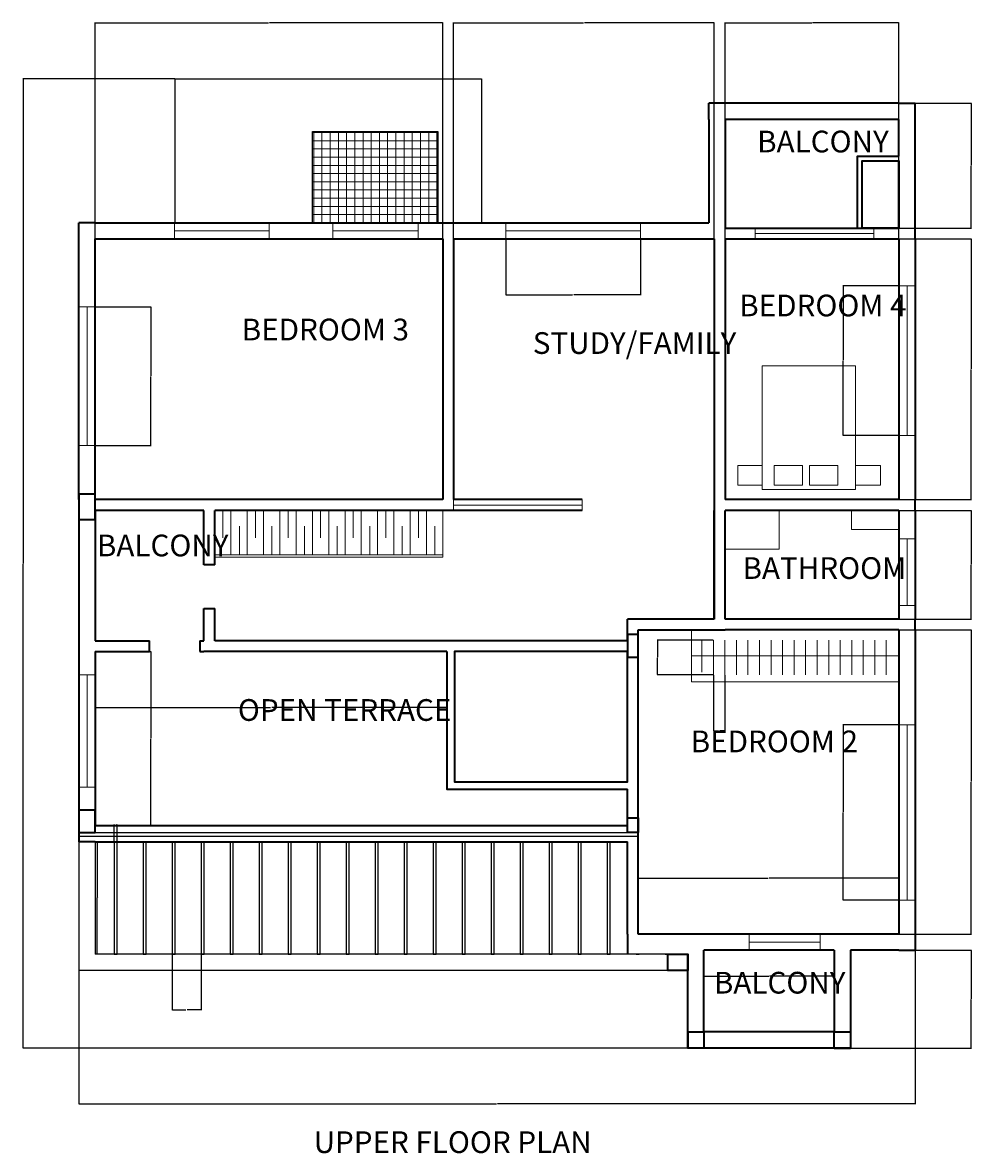
# Model space of a CAD drawing. Units: inches. Extents: x 1741 to 3812, y 9290 to 10023.
# Tile 3 of 5: x 2396 to 2921, y 9307 to 9932. Entities that reach past the tile are written whole.
import ezdxf

# ---------------------------------------------------------------- set-up
doc = ezdxf.new("R2010")
doc.units = ezdxf.units.IN
doc.header["$MEASUREMENT"] = 0
for name, color, linetype, lineweight in [('A-ANNO-DIMS', 2, 'Continuous', 18), ('A-ANNO-TEXT', 7, 'Continuous', 25), ('A-AREA-IDEN', 7, 'Continuous', 18), ('A-COLS', 1, 'Continuous', 35), ('A-FLOR-CASE', 9, 'Continuous', 18), ('A-FLOR-FIXT', 8, 'Continuous', 18), ('A-FLOR-STRS', 3, 'Continuous', 18), ('A-FURN', 9, 'Continuous', 18), ('A-GLAZ', 4, 'Continuous', 18), ('A-ROOF', 7, 'Continuous', 25), ('A-ROOF-PATT', 8, 'Continuous', 13), ('A-WALL', 7, 'Continuous', 35)]:
    doc.layers.add(name, color=color, linetype=linetype, lineweight=lineweight)
doc.styles.get("Standard").update_dxf_attribs({"font": 'arial.ttf'})
doc.dimstyles.get("Standard").update_dxf_attribs({"dimtxt": 0.18, "dimasz": 0.18, "dimexe": 0.18, "dimexo": 0.0625, "dimgap": 0.09, "dimtad": 0, "dimtih": 1, "dimtoh": 1, "dimdec": 4, "dimzin": 0, "dimdsep": 46, "dimtxsty": 'Standard', "dimcen": 0.09, "dimadec": 0, "dimazin": 0, "dimtfac": 1, "dimtdec": 4, "dimtofl": 0, "dimtmove": 0, "dimatfit": 3, "dimfxl": 1, "dimtolj": 1, "dimtzin": 0, "dimarcsym": 0})

# ---------------------------------------------------------------- blocks, each defined once
blk = doc.blocks.new('TERRACE-CANOPY-SLAT')
blk.add_lwpolyline([(0, 0), (1.8, 0), (1.8, 62.15), (0, 62.15)], close=True)
blk = doc.blocks.new('POST-9X9-PLAN')
blk.add_lwpolyline([(9, 0), (0, 0), (0, 9), (9, 9)], close=True)
blk = doc.blocks.new('WARDROBE-HANGER-PLAN')
for q in [(0, 0), (0, 1.59)]:
    blk.add_line((0, 19.29), q)
blk = doc.blocks.new('*D13')
at = {"layer": 'A-ANNO-DIMS', "color": 0, "lineweight": -2, "transparency": 16777216}
for p, q in [((2446.89, 9479.06), (2437.45, 9479.06)), ((2437.63, 9478.88), (2437.63, 9448.17)), ((2437.63, 9417.09), (2437.63, 9447.8)), ((2446.89, 9416.91), (2437.45, 9416.91))]:
    blk.add_line(p, q, dxfattribs=at)
at = {"layer": 'A-ANNO-DIMS', "color": 0, "transparency": 16777216}
for points in [[(2437.6, 9478.88), (2437.66, 9478.88), (2437.63, 9479.06)], [(2437.6, 9417.09), (2437.66, 9417.09), (2437.63, 9416.91)]]:
    blk.add_solid(points, dxfattribs=at)
at = {"layer": 'Defpoints', "color": 0, "transparency": 16777216}
for p in [(2437.63, 9479.06), (2446.95, 9479.06), (2446.95, 9416.91)]:
    blk.add_point(p, dxfattribs=at)
at = {"layer": 'A-ANNO-DIMS', "color": 0, "transparency": 16777216, "insert": (2437.63, 9447.98), "char_height": 0.18, "attachment_point": 5}
blk.add_mtext('\\A1;SLAT 62 TYP.', dxfattribs=at)
blk = doc.blocks.new('*D14')
at = {"layer": 'A-ANNO-DIMS', "color": 0, "lineweight": -2, "transparency": 16777216}
for p, q in [((2446.95, 9479.12), (2446.95, 9488.56)), ((2447.13, 9488.38), (2447.39, 9488.38)), ((2448.56, 9488.38), (2448.31, 9488.38)), ((2448.74, 9479.12), (2448.74, 9488.56))]:
    blk.add_line(p, q, dxfattribs=at)
at = {"layer": 'A-ANNO-DIMS', "color": 0, "transparency": 16777216}
for points in [[(2447.13, 9488.41), (2447.13, 9488.35), (2446.95, 9488.38)], [(2448.56, 9488.41), (2448.56, 9488.35), (2448.74, 9488.38)]]:
    blk.add_solid(points, dxfattribs=at)
at = {"layer": 'Defpoints', "color": 0, "transparency": 16777216}
for p in [(2448.74, 9488.38), (2446.95, 9479.06), (2448.74, 9479.06)]:
    blk.add_point(p, dxfattribs=at)
at = {"layer": 'A-ANNO-DIMS', "color": 0, "transparency": 16777216, "insert": (2447.85, 9488.38), "char_height": 0.18, "attachment_point": 5}
blk.add_mtext('\\A1;2 TYP.', dxfattribs=at)
blk = doc.blocks.new('*D56')
at = {"layer": 'A-ANNO-DIMS', "color": 0, "lineweight": -2, "transparency": 16777216}
for p, q in [((2889.54, 9419), (2889.54, 9334.08)), ((2427.54, 9407.89), (2427.54, 9334.08)), ((2427.72, 9334.26), (2658.25, 9334.26)), ((2889.36, 9334.26), (2658.83, 9334.26))]:
    blk.add_line(p, q, dxfattribs=at)
at = {"layer": 'A-ANNO-DIMS', "color": 0, "transparency": 16777216}
for points in [[(2427.72, 9334.29), (2427.72, 9334.23), (2427.54, 9334.26)], [(2889.36, 9334.29), (2889.36, 9334.23), (2889.54, 9334.26)]]:
    blk.add_solid(points, dxfattribs=at)
at = {"layer": 'Defpoints', "color": 0, "transparency": 16777216}
for p in [(2889.54, 9419.06), (2427.54, 9407.95), (2889.54, 9334.26)]:
    blk.add_point(p, dxfattribs=at)
at = {"layer": 'A-ANNO-DIMS', "color": 0, "transparency": 16777216, "insert": (2658.54, 9334.26), "char_height": 0.18, "attachment_point": 5}
blk.add_mtext('\\A1;462', dxfattribs=at)
blk = doc.blocks.new('*D57')
at = {"layer": 'A-ANNO-DIMS', "color": 0, "lineweight": -2, "transparency": 16777216}
for p, q in [((2480.59, 9900.6), (2396.56, 9900.6)), ((2396.74, 9900.42), (2396.74, 9633.01)), ((2396.74, 9365.24), (2396.74, 9632.65)), ((2763.77, 9365.06), (2396.56, 9365.06))]:
    blk.add_line(p, q, dxfattribs=at)
at = {"layer": 'A-ANNO-DIMS', "color": 0, "transparency": 16777216}
for points in [[(2396.71, 9900.42), (2396.77, 9900.42), (2396.74, 9900.6)], [(2396.71, 9365.24), (2396.77, 9365.24), (2396.74, 9365.06)]]:
    blk.add_solid(points, dxfattribs=at)
at = {"layer": 'Defpoints', "color": 0, "transparency": 16777216}
for p in [(2396.74, 9900.6), (2480.65, 9900.6), (2763.83, 9365.06)]:
    blk.add_point(p, dxfattribs=at)
at = {"layer": 'A-ANNO-DIMS', "color": 0, "transparency": 16777216, "insert": (2396.74, 9632.83), "char_height": 0.18, "attachment_point": 5}
blk.add_mtext('\\A1;535.5', dxfattribs=at)
blk = doc.blocks.new('*D58')
at = {"layer": 'A-ANNO-DIMS', "color": 0, "lineweight": -2, "transparency": 16777216}
for p, q in [((2436.54, 9812.12), (2436.54, 9931.58)), ((2436.72, 9931.4), (2532.26, 9931.4)), ((2628.36, 9931.4), (2532.82, 9931.4)), ((2628.54, 9812.12), (2628.54, 9931.58))]:
    blk.add_line(p, q, dxfattribs=at)
at = {"layer": 'A-ANNO-DIMS', "color": 0, "transparency": 16777216}
for points in [[(2436.72, 9931.43), (2436.72, 9931.37), (2436.54, 9931.4)], [(2628.36, 9931.43), (2628.36, 9931.37), (2628.54, 9931.4)]]:
    blk.add_solid(points, dxfattribs=at)
at = {"layer": 'Defpoints', "color": 0, "transparency": 16777216}
for p in [(2628.54, 9931.4), (2436.54, 9812.06), (2628.54, 9812.06)]:
    blk.add_point(p, dxfattribs=at)
at = {"layer": 'A-ANNO-DIMS', "color": 0, "transparency": 16777216, "insert": (2532.54, 9931.4), "char_height": 0.18, "attachment_point": 5}
blk.add_mtext('\\A1;192', dxfattribs=at)
blk = doc.blocks.new('*D59')
at = {"layer": 'A-ANNO-DIMS', "color": 0, "lineweight": -2, "transparency": 16777216}
for p, q in [((2634.54, 9812.12), (2634.54, 9931.58)), ((2634.72, 9931.4), (2706.26, 9931.4)), ((2778.36, 9931.4), (2706.82, 9931.4)), ((2778.54, 9812.12), (2778.54, 9931.58))]:
    blk.add_line(p, q, dxfattribs=at)
at = {"layer": 'A-ANNO-DIMS', "color": 0, "transparency": 16777216}
for points in [[(2634.72, 9931.43), (2634.72, 9931.37), (2634.54, 9931.4)], [(2778.36, 9931.43), (2778.36, 9931.37), (2778.54, 9931.4)]]:
    blk.add_solid(points, dxfattribs=at)
at = {"layer": 'Defpoints', "color": 0, "transparency": 16777216}
for p in [(2778.54, 9931.4), (2634.54, 9812.06), (2778.54, 9812.06)]:
    blk.add_point(p, dxfattribs=at)
at = {"layer": 'A-ANNO-DIMS', "color": 0, "transparency": 16777216, "insert": (2706.54, 9931.4), "char_height": 0.18, "attachment_point": 5}
blk.add_mtext('\\A1;144', dxfattribs=at)
blk = doc.blocks.new('*D60')
at = {"layer": 'A-ANNO-DIMS', "color": 0, "lineweight": -2, "transparency": 16777216}
for p, q in [((2784.54, 9812.12), (2784.54, 9931.58)), ((2784.72, 9931.4), (2832.32, 9931.4)), ((2880.36, 9931.4), (2832.76, 9931.4)), ((2880.54, 9812.12), (2880.54, 9931.58))]:
    blk.add_line(p, q, dxfattribs=at)
at = {"layer": 'A-ANNO-DIMS', "color": 0, "transparency": 16777216}
for points in [[(2784.72, 9931.43), (2784.72, 9931.37), (2784.54, 9931.4)], [(2880.36, 9931.43), (2880.36, 9931.37), (2880.54, 9931.4)]]:
    blk.add_solid(points, dxfattribs=at)
at = {"layer": 'Defpoints', "color": 0, "transparency": 16777216}
for p in [(2880.54, 9931.4), (2784.54, 9812.06), (2880.54, 9812.06)]:
    blk.add_point(p, dxfattribs=at)
at = {"layer": 'A-ANNO-DIMS', "color": 0, "transparency": 16777216, "insert": (2832.54, 9931.4), "char_height": 0.18, "attachment_point": 5}
blk.add_mtext('\\A1;96', dxfattribs=at)
blk = doc.blocks.new('*D61')
at = {"layer": 'A-ANNO-DIMS', "color": 0, "lineweight": -2, "transparency": 16777216}
for p, q in [((2889.6, 9887.06), (2920.52, 9887.06)), ((2920.34, 9886.88), (2920.34, 9852.74)), ((2920.34, 9818.24), (2920.34, 9852.38)), ((2880.6, 9818.06), (2920.52, 9818.06))]:
    blk.add_line(p, q, dxfattribs=at)
at = {"layer": 'A-ANNO-DIMS', "color": 0, "transparency": 16777216}
for points in [[(2920.31, 9886.88), (2920.37, 9886.88), (2920.34, 9887.06)], [(2920.31, 9818.24), (2920.37, 9818.24), (2920.34, 9818.06)]]:
    blk.add_solid(points, dxfattribs=at)
at = {"layer": 'Defpoints', "color": 0, "transparency": 16777216}
for p in [(2889.54, 9887.06), (2880.54, 9818.06), (2920.34, 9818.06)]:
    blk.add_point(p, dxfattribs=at)
at = {"layer": 'A-ANNO-DIMS', "color": 0, "transparency": 16777216, "insert": (2920.34, 9852.56), "char_height": 0.18, "attachment_point": 5}
blk.add_mtext('\\A1;69', dxfattribs=at)
blk = doc.blocks.new('*D62')
at = {"layer": 'A-ANNO-DIMS', "color": 0, "lineweight": -2, "transparency": 16777216}
for p, q in [((2880.6, 9812.06), (2920.52, 9812.06)), ((2920.34, 9811.88), (2920.34, 9740.24)), ((2920.34, 9668.24), (2920.34, 9739.88)), ((2880.6, 9668.06), (2920.52, 9668.06))]:
    blk.add_line(p, q, dxfattribs=at)
at = {"layer": 'A-ANNO-DIMS', "color": 0, "transparency": 16777216}
for points in [[(2920.31, 9811.88), (2920.37, 9811.88), (2920.34, 9812.06)], [(2920.31, 9668.24), (2920.37, 9668.24), (2920.34, 9668.06)]]:
    blk.add_solid(points, dxfattribs=at)
at = {"layer": 'Defpoints', "color": 0, "transparency": 16777216}
for p in [(2880.54, 9812.06), (2880.54, 9668.06), (2920.34, 9668.06)]:
    blk.add_point(p, dxfattribs=at)
at = {"layer": 'A-ANNO-DIMS', "color": 0, "transparency": 16777216, "insert": (2920.34, 9740.06), "char_height": 0.18, "attachment_point": 5}
blk.add_mtext('\\A1;144', dxfattribs=at)
blk = doc.blocks.new('*D63')
at = {"layer": 'A-ANNO-DIMS', "color": 0, "lineweight": -2, "transparency": 16777216}
for p, q in [((2880.6, 9662.06), (2920.52, 9662.06)), ((2920.34, 9661.88), (2920.34, 9632.24)), ((2920.34, 9602.24), (2920.34, 9631.88)), ((2880.6, 9602.06), (2920.52, 9602.06))]:
    blk.add_line(p, q, dxfattribs=at)
at = {"layer": 'A-ANNO-DIMS', "color": 0, "transparency": 16777216}
for points in [[(2920.31, 9661.88), (2920.37, 9661.88), (2920.34, 9662.06)], [(2920.31, 9602.24), (2920.37, 9602.24), (2920.34, 9602.06)]]:
    blk.add_solid(points, dxfattribs=at)
at = {"layer": 'Defpoints', "color": 0, "transparency": 16777216}
for p in [(2880.54, 9662.06), (2880.54, 9602.06), (2920.34, 9602.06)]:
    blk.add_point(p, dxfattribs=at)
at = {"layer": 'A-ANNO-DIMS', "color": 0, "transparency": 16777216, "insert": (2920.34, 9632.06), "char_height": 0.18, "attachment_point": 5}
blk.add_mtext('\\A1;60', dxfattribs=at)
blk = doc.blocks.new('*D64')
at = {"layer": 'A-ANNO-DIMS', "color": 0, "lineweight": -2, "transparency": 16777216}
for p, q in [((2880.6, 9596.06), (2920.52, 9596.06)), ((2920.34, 9595.88), (2920.34, 9512.24)), ((2920.34, 9428.24), (2920.34, 9511.88)), ((2880.6, 9428.06), (2920.52, 9428.06))]:
    blk.add_line(p, q, dxfattribs=at)
at = {"layer": 'A-ANNO-DIMS', "color": 0, "transparency": 16777216}
for points in [[(2920.31, 9595.88), (2920.37, 9595.88), (2920.34, 9596.06)], [(2920.31, 9428.24), (2920.37, 9428.24), (2920.34, 9428.06)]]:
    blk.add_solid(points, dxfattribs=at)
at = {"layer": 'Defpoints', "color": 0, "transparency": 16777216}
for p in [(2880.54, 9596.06), (2880.54, 9428.06), (2920.34, 9428.06)]:
    blk.add_point(p, dxfattribs=at)
at = {"layer": 'A-ANNO-DIMS', "color": 0, "transparency": 16777216, "insert": (2920.34, 9512.06), "char_height": 0.18, "attachment_point": 5}
blk.add_mtext('\\A1;168', dxfattribs=at)
blk = doc.blocks.new('*D65')
at = {"layer": 'A-ANNO-DIMS', "color": 0, "lineweight": -2, "transparency": 16777216}
for p, q in [((2853.89, 9419.06), (2920.52, 9419.06)), ((2920.34, 9418.88), (2920.34, 9392.24)), ((2920.34, 9365.24), (2920.34, 9391.88)), ((2853.89, 9365.06), (2920.52, 9365.06))]:
    blk.add_line(p, q, dxfattribs=at)
at = {"layer": 'A-ANNO-DIMS', "color": 0, "transparency": 16777216}
for points in [[(2920.31, 9418.88), (2920.37, 9418.88), (2920.34, 9419.06)], [(2920.31, 9365.24), (2920.37, 9365.24), (2920.34, 9365.06)]]:
    blk.add_solid(points, dxfattribs=at)
at = {"layer": 'Defpoints', "color": 0, "transparency": 16777216}
for p in [(2853.83, 9419.06), (2853.83, 9365.06), (2920.34, 9365.06)]:
    blk.add_point(p, dxfattribs=at)
at = {"layer": 'A-ANNO-DIMS', "color": 0, "transparency": 16777216, "insert": (2920.34, 9392.06), "char_height": 0.18, "attachment_point": 5}
blk.add_mtext('\\A1;54', dxfattribs=at)
blk = doc.blocks.new('*D66')
at = {"layer": 'A-ANNO-DIMS', "color": 0, "lineweight": -2, "transparency": 16777216}
for p, q in [((2736.54, 9428.12), (2736.54, 9459.04)), ((2736.72, 9458.86), (2808.26, 9458.86)), ((2880.36, 9458.86), (2808.82, 9458.86)), ((2880.54, 9428.12), (2880.54, 9459.04))]:
    blk.add_line(p, q, dxfattribs=at)
at = {"layer": 'A-ANNO-DIMS', "color": 0, "transparency": 16777216}
for points in [[(2736.72, 9458.89), (2736.72, 9458.83), (2736.54, 9458.86)], [(2880.36, 9458.89), (2880.36, 9458.83), (2880.54, 9458.86)]]:
    blk.add_solid(points, dxfattribs=at)
at = {"layer": 'Defpoints', "color": 0, "transparency": 16777216}
for p in [(2880.54, 9458.86), (2736.54, 9428.06), (2880.54, 9428.06)]:
    blk.add_point(p, dxfattribs=at)
at = {"layer": 'A-ANNO-DIMS', "color": 0, "transparency": 16777216, "insert": (2808.54, 9458.86), "char_height": 0.18, "attachment_point": 5}
blk.add_mtext('\\A1;144', dxfattribs=at)
blk = doc.blocks.new('*D67')
at = {"layer": 'A-ANNO-DIMS', "color": 0, "lineweight": -2, "transparency": 16777216}
for p, q in [((2436.6, 9584.06), (2467.52, 9584.06)), ((2467.34, 9583.88), (2467.34, 9536.24)), ((2467.34, 9488.24), (2467.34, 9535.88)), ((2436.6, 9488.06), (2467.52, 9488.06))]:
    blk.add_line(p, q, dxfattribs=at)
at = {"layer": 'A-ANNO-DIMS', "color": 0, "transparency": 16777216}
for points in [[(2467.31, 9583.88), (2467.37, 9583.88), (2467.34, 9584.06)], [(2467.31, 9488.24), (2467.37, 9488.24), (2467.34, 9488.06)]]:
    blk.add_solid(points, dxfattribs=at)
at = {"layer": 'Defpoints', "color": 0, "transparency": 16777216}
for p in [(2436.54, 9584.06), (2436.54, 9488.06), (2467.34, 9488.06)]:
    blk.add_point(p, dxfattribs=at)
at = {"layer": 'A-ANNO-DIMS', "color": 0, "transparency": 16777216, "insert": (2467.34, 9536.06), "char_height": 0.18, "attachment_point": 5}
blk.add_mtext('\\A1;96', dxfattribs=at)
blk = doc.blocks.new('*D68')
at = {"layer": 'A-ANNO-DIMS', "color": 0, "lineweight": -2, "transparency": 16777216}
for p, q in [((2772.83, 9374.12), (2772.83, 9405.04)), ((2773.01, 9404.86), (2808.61, 9404.86)), ((2844.65, 9404.86), (2809.05, 9404.86)), ((2844.83, 9374.12), (2844.83, 9405.04))]:
    blk.add_line(p, q, dxfattribs=at)
at = {"layer": 'A-ANNO-DIMS', "color": 0, "transparency": 16777216}
for points in [[(2773.01, 9404.89), (2773.01, 9404.83), (2772.83, 9404.86)], [(2844.65, 9404.89), (2844.65, 9404.83), (2844.83, 9404.86)]]:
    blk.add_solid(points, dxfattribs=at)
at = {"layer": 'Defpoints', "color": 0, "transparency": 16777216}
for p in [(2844.83, 9404.86), (2772.83, 9374.06), (2844.83, 9374.06)]:
    blk.add_point(p, dxfattribs=at)
at = {"layer": 'A-ANNO-DIMS', "color": 0, "transparency": 16777216, "insert": (2808.83, 9404.86), "char_height": 0.18, "attachment_point": 5}
blk.add_mtext('\\A1;72', dxfattribs=at)
blk = doc.blocks.new('*D69')
at = {"layer": 'A-ANNO-DIMS', "color": 0, "lineweight": -2, "transparency": 16777216}
for p, q in [((2777.97, 9590.5), (2747.05, 9590.5)), ((2747.23, 9590.32), (2747.23, 9581.03)), ((2747.23, 9571.39), (2747.23, 9580.67)), ((2777.97, 9571.21), (2747.05, 9571.21))]:
    blk.add_line(p, q, dxfattribs=at)
at = {"layer": 'A-ANNO-DIMS', "color": 0, "transparency": 16777216}
for points in [[(2747.2, 9590.32), (2747.26, 9590.32), (2747.23, 9590.5)], [(2747.2, 9571.39), (2747.26, 9571.39), (2747.23, 9571.21)]]:
    blk.add_solid(points, dxfattribs=at)
at = {"layer": 'Defpoints', "color": 0, "transparency": 16777216}
for p in [(2747.23, 9590.5), (2778.03, 9590.5), (2778.03, 9571.21)]:
    blk.add_point(p, dxfattribs=at)
at = {"layer": 'A-ANNO-DIMS', "color": 0, "transparency": 16777216, "insert": (2747.23, 9580.85), "char_height": 0.18, "attachment_point": 5}
blk.add_mtext('\\A1;19.29', dxfattribs=at)
blk = doc.blocks.new('*D70')
at = {"layer": 'A-ANNO-DIMS', "color": 0, "lineweight": -2, "transparency": 16777216}
for p, q in [((2778.03, 9571.15), (2778.03, 9540.23)), ((2784.4, 9571.15), (2784.4, 9540.23)), ((2778.21, 9540.41), (2780.82, 9540.41)), ((2784.22, 9540.41), (2781.61, 9540.41))]:
    blk.add_line(p, q, dxfattribs=at)
at = {"layer": 'A-ANNO-DIMS', "color": 0, "transparency": 16777216}
for points in [[(2778.21, 9540.44), (2778.21, 9540.38), (2778.03, 9540.41)], [(2784.22, 9540.44), (2784.22, 9540.38), (2784.4, 9540.41)]]:
    blk.add_solid(points, dxfattribs=at)
at = {"layer": 'Defpoints', "color": 0, "transparency": 16777216}
for p in [(2778.03, 9571.21), (2784.4, 9571.21), (2778.03, 9540.41)]:
    blk.add_point(p, dxfattribs=at)
at = {"layer": 'A-ANNO-DIMS', "color": 0, "transparency": 16777216, "insert": (2781.21, 9540.41), "char_height": 0.18, "attachment_point": 5}
blk.add_mtext('\\A1;6.369', dxfattribs=at)
blk = doc.blocks.new('*D71')
at = {"layer": 'A-ANNO-DIMS', "color": 0, "lineweight": -2, "transparency": 16777216}
for p, q in [((2478.99, 9416.85), (2478.99, 9385.93)), ((2495.01, 9416.85), (2495.01, 9385.93)), ((2479.17, 9386.11), (2486.61, 9386.11)), ((2494.83, 9386.11), (2487.38, 9386.11))]:
    blk.add_line(p, q, dxfattribs=at)
at = {"layer": 'A-ANNO-DIMS', "color": 0, "transparency": 16777216}
for points in [[(2479.17, 9386.14), (2479.17, 9386.08), (2478.99, 9386.11)], [(2494.83, 9386.14), (2494.83, 9386.08), (2495.01, 9386.11)]]:
    blk.add_solid(points, dxfattribs=at)
at = {"layer": 'Defpoints', "color": 0, "transparency": 16777216}
for p in [(2478.99, 9416.91), (2495.01, 9416.91), (2478.99, 9386.11)]:
    blk.add_point(p, dxfattribs=at)
at = {"layer": 'A-ANNO-DIMS', "color": 0, "transparency": 16777216, "insert": (2487, 9386.11), "char_height": 0.18, "attachment_point": 5}
blk.add_mtext('\\A1;16.02', dxfattribs=at)
blk = doc.blocks.new('*D72')
at = {"layer": 'A-ANNO-DIMS', "color": 0, "lineweight": -2, "transparency": 16777216}
for p, q in [((2436.54, 9584), (2436.54, 9553.08)), ((2630.85, 9584), (2630.85, 9553.08)), ((2436.72, 9553.26), (2533.31, 9553.26)), ((2630.67, 9553.26), (2534.08, 9553.26))]:
    blk.add_line(p, q, dxfattribs=at)
at = {"layer": 'A-ANNO-DIMS', "color": 0, "transparency": 16777216}
for points in [[(2436.72, 9553.29), (2436.72, 9553.23), (2436.54, 9553.26)], [(2630.67, 9553.29), (2630.67, 9553.23), (2630.85, 9553.26)]]:
    blk.add_solid(points, dxfattribs=at)
at = {"layer": 'Defpoints', "color": 0, "transparency": 16777216}
for p in [(2436.54, 9584.06), (2630.85, 9584.06), (2436.54, 9553.26)]:
    blk.add_point(p, dxfattribs=at)
at = {"layer": 'A-ANNO-DIMS', "color": 0, "transparency": 16777216, "insert": (2533.69, 9553.26), "char_height": 0.18, "attachment_point": 5}
blk.add_mtext('\\A1;194.3', dxfattribs=at)
blk = doc.blocks.new('*D73')
at = {"layer": 'A-ANNO-DIMS', "color": 0, "lineweight": -2, "transparency": 16777216}
for p, q in [((2436.6, 9774.48), (2467.52, 9774.48)), ((2467.34, 9774.3), (2467.34, 9736.38)), ((2467.34, 9698.1), (2467.34, 9736.02)), ((2436.6, 9697.92), (2467.52, 9697.92))]:
    blk.add_line(p, q, dxfattribs=at)
at = {"layer": 'A-ANNO-DIMS', "color": 0, "transparency": 16777216}
for points in [[(2467.31, 9774.3), (2467.37, 9774.3), (2467.34, 9774.48)], [(2467.31, 9698.1), (2467.37, 9698.1), (2467.34, 9697.92)]]:
    blk.add_solid(points, dxfattribs=at)
at = {"layer": 'Defpoints', "color": 0, "transparency": 16777216}
for p in [(2436.54, 9774.48), (2436.54, 9697.92), (2467.34, 9697.92)]:
    blk.add_point(p, dxfattribs=at)
at = {"layer": 'A-ANNO-DIMS', "color": 0, "transparency": 16777216, "insert": (2467.34, 9736.2), "char_height": 0.18, "attachment_point": 5}
blk.add_mtext('\\A1;76.57', dxfattribs=at)
blk = doc.blocks.new('*D74')
at = {"layer": 'A-ANNO-DIMS', "color": 0, "lineweight": -2, "transparency": 16777216}
for p, q in [((2663.36, 9812), (2663.36, 9781.08)), ((2737.76, 9812), (2737.76, 9781.08)), ((2663.54, 9781.26), (2700.24, 9781.26)), ((2737.58, 9781.26), (2700.88, 9781.26))]:
    blk.add_line(p, q, dxfattribs=at)
at = {"layer": 'A-ANNO-DIMS', "color": 0, "transparency": 16777216}
for points in [[(2663.54, 9781.29), (2663.54, 9781.23), (2663.36, 9781.26)], [(2737.58, 9781.29), (2737.58, 9781.23), (2737.76, 9781.26)]]:
    blk.add_solid(points, dxfattribs=at)
at = {"layer": 'Defpoints', "color": 0, "transparency": 16777216}
for p in [(2663.36, 9812.06), (2737.76, 9812.06), (2663.36, 9781.26)]:
    blk.add_point(p, dxfattribs=at)
at = {"layer": 'A-ANNO-DIMS', "color": 0, "transparency": 16777216, "insert": (2700.56, 9781.26), "char_height": 0.18, "attachment_point": 5}
blk.add_mtext('\\A1;74.4', dxfattribs=at)
blk = doc.blocks.new('*D75')
at = {"layer": 'A-ANNO-DIMS', "color": 0, "lineweight": -2, "transparency": 16777216}
for p, q in [((2880.48, 9786.2), (2849.56, 9786.2)), ((2849.74, 9786.02), (2849.74, 9745.05)), ((2849.74, 9703.72), (2849.74, 9744.69)), ((2880.48, 9703.54), (2849.56, 9703.54))]:
    blk.add_line(p, q, dxfattribs=at)
at = {"layer": 'A-ANNO-DIMS', "color": 0, "transparency": 16777216}
for points in [[(2849.71, 9786.02), (2849.77, 9786.02), (2849.74, 9786.2)], [(2849.71, 9703.72), (2849.77, 9703.72), (2849.74, 9703.54)]]:
    blk.add_solid(points, dxfattribs=at)
at = {"layer": 'Defpoints', "color": 0, "transparency": 16777216}
for p in [(2849.74, 9786.2), (2880.54, 9786.2), (2880.54, 9703.54)]:
    blk.add_point(p, dxfattribs=at)
at = {"layer": 'A-ANNO-DIMS', "color": 0, "transparency": 16777216, "insert": (2849.74, 9744.87), "char_height": 0.18, "attachment_point": 5}
blk.add_mtext('\\A1;82.66', dxfattribs=at)
blk = doc.blocks.new('*D76')
at = {"layer": 'A-ANNO-DIMS', "color": 0, "lineweight": -2, "transparency": 16777216}
for p, q in [((2880.48, 9543.69), (2849.56, 9543.69)), ((2849.74, 9543.51), (2849.74, 9495.44)), ((2849.74, 9447.01), (2849.74, 9495.08)), ((2880.48, 9446.83), (2849.56, 9446.83))]:
    blk.add_line(p, q, dxfattribs=at)
at = {"layer": 'A-ANNO-DIMS', "color": 0, "transparency": 16777216}
for points in [[(2849.71, 9543.51), (2849.77, 9543.51), (2849.74, 9543.69)], [(2849.71, 9447.01), (2849.77, 9447.01), (2849.74, 9446.83)]]:
    blk.add_solid(points, dxfattribs=at)
at = {"layer": 'Defpoints', "color": 0, "transparency": 16777216}
for p in [(2849.74, 9543.69), (2880.54, 9543.69), (2880.54, 9446.83)]:
    blk.add_point(p, dxfattribs=at)
at = {"layer": 'A-ANNO-DIMS', "color": 0, "transparency": 16777216, "insert": (2849.74, 9495.26), "char_height": 0.18, "attachment_point": 5}
blk.add_mtext('\\A1;96.86', dxfattribs=at)

msp = doc.modelspace()

# ---------------------------------------------------------------- hatches: boundary and pattern name
at = {"layer": 'A-ROOF-PATT'}
h = msp.add_hatch(dxfattribs=at)
h.set_pattern_fill('NET', color=256, scale=36.27322, style=0)
h.paths.add_polyline_path([(2556.6539, 9821.0599), (2625.8165, 9821.0599), (2625.8165, 9871.3807), (2556.6539, 9871.3807)])

# ---------------------------------------------------------------- linework, layer by layer
at = {"layer": 'A-COLS'}
for points in [[(2436.5397, 9671.0807), (2427.5397, 9671.0807), (2427.5397, 9657.1373), (2436.5397, 9657.1373)], [(2736.5397, 9593.6037), (2730.5397, 9593.6037), (2730.5397, 9581.0445), (2736.5397, 9581.0445)], [(2427.5397, 9484.1652), (2436.5397, 9484.1652), (2436.5397, 9496.5144), (2427.5397, 9496.5144)], [(2736.5397, 9484.1652), (2730.5397, 9484.1652), (2730.5397, 9492.1899), (2736.5397, 9492.1899)], [(2752.9474, 9416.9087), (2763.8294, 9416.9087), (2763.8294, 9407.9488), (2752.9474, 9407.9488)]]:
    msp.add_lwpolyline(points, close=True, dxfattribs=at)
at = {"layer": 'A-FLOR-CASE'}
for p, q in [((2771.6603, 9590.4984), (2771.6603, 9572.7985)), ((2873.56, 9590.4984), (2873.56, 9571.2075)), ((2765.8732, 9581.7591), (2880.5397, 9581.7591))]:
    msp.add_line(p, q, dxfattribs=at)
msp.add_lwpolyline([(2880.5397, 9596.0599), (2765.8732, 9596.0599), (2765.8732, 9567.4583), (2880.5397, 9567.4583)], close=True, dxfattribs=at)
at = {"layer": 'A-FLOR-FIXT'}
for points in [[(2784.5397, 9662.0599), (2814.3052, 9662.0599), (2814.3052, 9640.7182), (2784.5397, 9640.7182)], [(2880.5397, 9662.0599), (2854.3687, 9662.0599), (2854.3687, 9651.6074), (2880.5397, 9651.6074)]]:
    msp.add_lwpolyline(points, close=True, dxfattribs=at)
at = {"layer": 'A-FLOR-STRS'}
for p, q in [((2628.5397, 9662.0599), (2502.5397, 9662.0599)), ((2502.5397, 9662.0599), (2502.5397, 9637.5296)), ((2507.0408, 9662.0599), (2507.0408, 9646.8636)), ((2511.5397, 9662.0599), (2511.5397, 9637.5296)), ((2520.5397, 9662.0599), (2520.5397, 9637.5296)), ((2525.0408, 9662.0599), (2525.0408, 9646.8636)), ((2529.5397, 9662.0599), (2529.5397, 9637.5296)), ((2538.5397, 9662.0599), (2538.5397, 9637.5296)), ((2543.0408, 9662.0599), (2543.0408, 9646.8636)), ((2547.5397, 9662.0599), (2547.5397, 9637.5296)), ((2556.5397, 9662.0599), (2556.5397, 9637.5296)), ((2561.0408, 9662.0599), (2561.0408, 9646.8636)), ((2565.5397, 9662.0599), (2565.5397, 9637.5296)), ((2574.5397, 9662.0599), (2574.5397, 9637.5296)), ((2579.0408, 9662.0599), (2579.0408, 9646.8636)), ((2583.5397, 9662.0599), (2583.5397, 9637.5296)), ((2592.5397, 9662.0599), (2592.5397, 9637.5296)), ((2597.0408, 9662.0599), (2597.0408, 9646.8636)), ((2601.5397, 9662.0599), (2601.5397, 9637.5296)), ((2610.5397, 9662.0599), (2610.5397, 9637.5296)), ((2615.0408, 9662.0599), (2615.0408, 9646.8636)), ((2619.5397, 9662.0599), (2619.5397, 9637.5296)), ((2628.5397, 9637.5296), (2628.5397, 9662.0599)), ((2628.5397, 9662.0599), (2628.5397, 9636.2823)), ((2516.1834, 9637.5296), (2516.1834, 9653.3002)), ((2534.1834, 9637.5296), (2534.1834, 9653.3002)), ((2552.1834, 9637.5296), (2552.1834, 9653.3002)), ((2570.1834, 9637.5296), (2570.1834, 9653.3002)), ((2588.1834, 9637.5296), (2588.1834, 9653.3002)), ((2606.1834, 9637.5296), (2606.1834, 9653.3002)), ((2624.1834, 9637.5296), (2624.1834, 9653.3002)), ((2502.5397, 9637.5296), (2628.5397, 9637.5296)), ((2502.5397, 9636.2823), (2628.5397, 9636.2823))]:
    msp.add_line(p, q, dxfattribs=at)
at = {"layer": 'A-FURN'}
for points in [[(2805.0105, 9673.7062), (2856.6166, 9673.7062), (2856.6166, 9741.9619), (2805.0105, 9741.9619)], [(2811.5611, 9676.0539), (2827.3358, 9676.0539), (2827.3358, 9686.9744), (2811.5611, 9686.9744)], [(2831.0387, 9676.0539), (2846.8135, 9676.0539), (2846.8135, 9686.9744), (2831.0387, 9686.9744)]]:
    msp.add_lwpolyline(points, close=True, dxfattribs=at)
for points in [[(2805.0105, 9686.9744), (2791.451, 9686.9744), (2791.451, 9676.0539), (2805.0105, 9676.0539)], [(2856.6166, 9676.0539), (2870.3384, 9676.0539), (2870.3384, 9686.9744), (2856.6166, 9686.9744)]]:
    msp.add_lwpolyline(points, dxfattribs=at)
at = {"layer": 'A-GLAZ'}
for p, q in [((2480.2578, 9816.5599), (2532.5397, 9816.5599)), ((2567.8825, 9816.5599), (2615.0013, 9816.5599)), ((2663.3602, 9816.5599), (2737.7585, 9816.5599)), ((2885.0397, 9703.5403), (2885.0397, 9786.197)), ((2432.0397, 9774.4824), (2432.0397, 9697.9157)), ((2634.5397, 9665.0599), (2705.4442, 9665.0599)), ((2885.0397, 9646.4038), (2885.0397, 9609.5179)), ((2432.0397, 9571.3216), (2432.0397, 9509.1765)), ((2885.0397, 9543.6909), (2885.0397, 9446.8276)), ((2797.7718, 9423.5599), (2836.9401, 9423.5599))]:
    msp.add_line(p, q, dxfattribs=at)
for points in [[(2480.2578, 9821.0599), (2532.5397, 9821.0599), (2532.5397, 9812.0599), (2480.2578, 9812.0599)], [(2615.0013, 9812.0599), (2567.8825, 9812.0599), (2567.8825, 9821.0599), (2615.0013, 9821.0599)], [(2663.3602, 9812.0599), (2737.7585, 9812.0599), (2737.7585, 9821.0599), (2663.3602, 9821.0599)], [(2801.079, 9812.0599), (2866.6472, 9812.0599), (2866.6472, 9818.0599), (2801.079, 9818.0599)], [(2801.079, 9815.0599), (2866.6472, 9815.0599), (2866.6472, 9815.0599), (2801.079, 9815.0599)], [(2889.5397, 9703.5403), (2880.5397, 9703.5403), (2880.5397, 9786.197), (2889.5397, 9786.197)], [(2436.5397, 9697.9157), (2427.5397, 9697.9157), (2427.5397, 9774.4824), (2436.5397, 9774.4824)], [(2634.5397, 9668.0599), (2705.4442, 9668.0599), (2705.4442, 9662.0599), (2634.5397, 9662.0599)], [(2889.5397, 9609.5179), (2880.5397, 9609.5179), (2880.5397, 9646.4038), (2889.5397, 9646.4038)], [(2436.5397, 9509.1765), (2427.5397, 9509.1765), (2427.5397, 9571.3216), (2436.5397, 9571.3216)], [(2889.5397, 9446.8276), (2880.5397, 9446.8276), (2880.5397, 9543.6909), (2889.5397, 9543.6909)], [(2836.9401, 9419.0599), (2797.7718, 9419.0599), (2797.7718, 9428.0599), (2836.9401, 9428.0599)]]:
    msp.add_lwpolyline(points, close=True, dxfattribs=at)
at = {"layer": 'A-ROOF'}
for p, q in [((2556.6539, 9871.3807), (2625.8165, 9871.3807)), ((2556.6539, 9821.0599), (2556.6539, 9871.3807)), ((2625.8165, 9871.3807), (2625.8165, 9821.0599)), ((2625.8165, 9821.0599), (2556.6539, 9821.0599)), ((2427.5397, 9479.0599), (2427.5397, 9407.9488)), ((2436.5397, 9479.0599), (2436.5397, 9416.9087)), ((2763.8294, 9416.9087), (2436.5397, 9416.9087)), ((2763.8294, 9407.9488), (2427.5397, 9407.9488))]:
    msp.add_line(p, q, dxfattribs=at)
for points in [[(2649.888, 9821.0599), (2480.6506, 9821.0599), (2480.6506, 9900.5994), (2649.888, 9900.5994)], [(2427.5397, 9484.1652), (2736.5397, 9484.1652), (2736.5397, 9482.0185), (2427.5397, 9482.0185)]]:
    msp.add_lwpolyline(points, close=True, dxfattribs=at)
for points in [[(2735.2955, 9416.9087), (2735.2955, 9416.9087), (2737.0921, 9416.9087)], [(2751.3147, 9416.9087), (2751.3147, 9416.9087), (2753.1114, 9416.9087)]]:
    msp.add_lwpolyline(points, dxfattribs=at)
at = {"layer": 'A-WALL'}
for p, q in [((2775.5397, 9878.0599), (2775.5397, 9887.0599)), ((2784.5397, 9887.0599), (2775.5397, 9887.0599)), ((2880.5397, 9887.0599), (2784.5397, 9887.0599)), ((2880.5397, 9887.0599), (2889.5397, 9887.0599)), ((2889.5397, 9878.0599), (2889.5397, 9887.0599)), ((2775.5397, 9878.0599), (2775.5397, 9821.0599)), ((2880.5397, 9878.0599), (2784.5397, 9878.0599)), ((2784.5397, 9878.0599), (2784.5397, 9818.0599)), ((2880.5397, 9857.8827), (2880.5397, 9878.0599)), ((2889.5397, 9818.0599), (2889.5397, 9878.0599)), ((2880.5397, 9818.0599), (2880.5397, 9855.273)), ((2436.5397, 9821.0599), (2427.5397, 9821.0599)), ((2427.5397, 9812.0599), (2427.5397, 9821.0599)), ((2436.5397, 9821.0599), (2775.5397, 9821.0599)), ((2634.5397, 9821.0599), (2775.5397, 9821.0599)), ((2784.5397, 9818.0599), (2880.5397, 9818.0599)), ((2889.5397, 9812.0599), (2889.5397, 9818.0599)), ((2427.5397, 9668.0599), (2427.5397, 9812.0599)), ((2436.5397, 9812.0599), (2628.5397, 9812.0599)), ((2436.5397, 9668.0599), (2436.5397, 9812.0599)), ((2628.5397, 9812.0599), (2628.5397, 9668.0599)), ((2634.5397, 9812.0599), (2634.5397, 9668.0599)), ((2634.5397, 9812.0599), (2778.5397, 9812.0599)), ((2778.5397, 9812.0599), (2778.5397, 9602.0599)), ((2784.5397, 9812.0599), (2784.5397, 9668.0599)), ((2784.5397, 9812.0599), (2880.5397, 9812.0599)), ((2880.5397, 9812.0599), (2880.5397, 9668.0599)), ((2889.5397, 9812.0599), (2889.5397, 9668.0599)), ((2427.5397, 9668.0599), (2427.5397, 9662.0599)), ((2628.5397, 9668.0599), (2436.5397, 9668.0599)), ((2705.4442, 9668.0599), (2634.5397, 9668.0599)), ((2880.5397, 9668.0599), (2784.5397, 9668.0599)), ((2889.5397, 9662.0599), (2889.5397, 9668.0599)), ((2427.5397, 9662.0599), (2427.5397, 9590.0599)), ((2436.5397, 9662.0599), (2436.5397, 9590.0599)), ((2496.5397, 9662.0599), (2436.5397, 9662.0599)), ((2496.5397, 9631.9948), (2496.5397, 9662.0599)), ((2628.5397, 9662.0599), (2502.5397, 9662.0599)), ((2705.4442, 9662.0599), (2502.5397, 9662.0599)), ((2502.5397, 9631.9948), (2502.5397, 9662.0599)), ((2778.5397, 9602.0599), (2778.5397, 9662.0599)), ((2880.5397, 9662.0599), (2784.5397, 9662.0599)), ((2784.5397, 9602.0599), (2784.5397, 9662.0599)), ((2880.5397, 9662.0599), (2880.5397, 9602.0599)), ((2889.5397, 9662.0599), (2889.5397, 9602.0599)), ((2496.5397, 9590.0599), (2496.5397, 9607.9205)), ((2502.5397, 9590.0599), (2502.5397, 9607.9205)), ((2730.5397, 9590.0599), (2730.5397, 9602.0599)), ((2778.5397, 9602.0599), (2730.5397, 9602.0599)), ((2880.5397, 9602.0599), (2784.5397, 9602.0599)), ((2889.5397, 9596.0599), (2889.5397, 9602.0599)), ((2736.5397, 9428.0599), (2736.5397, 9596.0599)), ((2736.5397, 9596.0599), (2784.5397, 9596.0599)), ((2880.5397, 9596.0599), (2784.5397, 9596.0599)), ((2880.5397, 9596.0599), (2880.5397, 9428.0599)), ((2889.5397, 9596.0599), (2889.5397, 9428.0599)), ((2427.5397, 9590.0599), (2427.5397, 9584.0599)), ((2436.5397, 9590.0599), (2466.5397, 9590.0599)), ((2494.3167, 9590.0599), (2496.5397, 9590.0599)), ((2730.5397, 9590.0599), (2502.5397, 9590.0599)), ((2427.5397, 9584.0599), (2427.5397, 9488.0599)), ((2436.5397, 9584.0599), (2466.5397, 9584.0599)), ((2436.5397, 9584.0599), (2436.5397, 9488.0599)), ((2494.3167, 9584.0599), (2496.5397, 9584.0599)), ((2630.8472, 9584.0599), (2496.5397, 9584.0599)), ((2730.5397, 9584.0599), (2635.0071, 9584.0599)), ((2730.5397, 9512.1654), (2730.5397, 9584.0599)), ((2730.5397, 9488.0599), (2730.5397, 9508.0055)), ((2427.5397, 9488.0599), (2427.5397, 9479.0599)), ((2436.5397, 9488.0599), (2730.5397, 9488.0599)), ((2436.5397, 9479.0599), (2427.5397, 9479.0599)), ((2436.5397, 9479.0599), (2730.5397, 9479.0599)), ((2730.5397, 9428.0599), (2730.5397, 9479.0599)), ((2730.5397, 9428.0599), (2730.5397, 9416.9087)), ((2880.5397, 9428.0599), (2736.5397, 9428.0599)), ((2889.5397, 9428.0599), (2889.5397, 9419.0599)), ((2763.8294, 9374.0599), (2763.8294, 9416.9087)), ((2772.8294, 9374.0599), (2772.8294, 9419.0599)), ((2844.8294, 9419.0599), (2772.8294, 9419.0599)), ((2844.8294, 9419.0599), (2844.8294, 9374.0599)), ((2853.8294, 9419.0599), (2853.8294, 9374.0599)), ((2880.5397, 9419.0599), (2853.8294, 9419.0599)), ((2880.5397, 9419.0599), (2889.5397, 9419.0599)), ((2763.8294, 9374.0599), (2763.8294, 9365.0599)), ((2844.8294, 9374.0599), (2772.8294, 9374.0599)), ((2853.8294, 9374.0599), (2853.8294, 9365.0599)), ((2772.8294, 9365.0599), (2763.8294, 9365.0599)), ((2844.8294, 9365.0599), (2772.8294, 9365.0599)), ((2844.8294, 9365.0599), (2853.8294, 9365.0599))]:
    msp.add_line(p, q, dxfattribs=at)
for points in [[(2857.6888, 9818.0599), (2857.6888, 9857.8827), (2880.5397, 9857.8827)], [(2502.5397, 9631.9948), (2496.5397, 9631.9948)], [(2496.5397, 9607.9205), (2502.5397, 9607.9205)], [(2466.5397, 9584.0599), (2466.5397, 9590.0599)], [(2494.3167, 9590.0599), (2494.3167, 9584.0599)], [(2630.8472, 9584.0599), (2630.8472, 9508.0055), (2730.5397, 9508.0055)]]:
    msp.add_lwpolyline(points, dxfattribs=at)
for points in [[(2880.5397, 9818.0599), (2860.2985, 9818.0599), (2860.2985, 9855.273), (2880.5397, 9855.273)], [(2730.5397, 9584.0599), (2635.0071, 9584.0599), (2635.0071, 9512.1654), (2730.5397, 9512.1654)]]:
    msp.add_lwpolyline(points, close=True, dxfattribs=at)

# ---------------------------------------------------------------- block references
at = {"layer": 'A-COLS'}
for p, rotation in [((2772.8291, 9365.0597), 90.00000000000479), ((2853.8295, 9374.0596), 180)]:
    msp.add_blockref('POST-9X9-PLAN', p, dxfattribs=dict(at, rotation=rotation))
at = {"layer": 'A-FLOR-CASE'}
for p in [(2778.029, 9571.208), (2784.3977, 9571.208), (2790.7665, 9571.208), (2797.1352, 9571.208), (2803.5039, 9571.208), (2809.8727, 9571.208), (2816.2414, 9571.208), (2822.6101, 9571.208), (2828.9789, 9571.208), (2835.3476, 9571.208), (2841.7163, 9571.208), (2848.0851, 9571.208), (2854.4538, 9571.208), (2860.8226, 9571.208), (2867.1913, 9571.208)]:
    msp.add_blockref('WARDROBE-HANGER-PLAN', p, dxfattribs=at)
at = {"layer": 'A-ROOF'}
for p in [(2446.948, 9416.909), (2462.9673, 9416.909), (2478.9866, 9416.909), (2495.0059, 9416.909), (2511.0251, 9416.909), (2527.0444, 9416.909), (2543.0637, 9416.909), (2559.083, 9416.909), (2575.1023, 9416.909), (2591.1216, 9416.909), (2607.1409, 9416.909), (2623.1602, 9416.909), (2639.1794, 9416.909), (2655.1987, 9416.909), (2671.218, 9416.909), (2687.2373, 9416.909), (2703.2566, 9416.909), (2719.2759, 9416.909)]:
    msp.add_blockref('TERRACE-CANOPY-SLAT', p, dxfattribs=at)

# ---------------------------------------------------------------- texts
at = {"layer": 'A-ANNO-TEXT'}
msp.add_text('UPPER FLOOR PLAN', height=12, dxfattribs=at).set_placement((2557.2179, 9307.093))
at = {"layer": 'A-AREA-IDEN'}
for s, p in [('BALCONY', (2802.1816, 9859.8778)), ('BEDROOM 4', (2792.3074, 9769.2958)), ('BEDROOM 3 ', (2517.4793, 9756.0136)), ('STUDY/FAMILY', (2678.2744, 9748.5536)), ('BALCONY ', (2437.4666, 9636.7207)), ('BATHROOM', (2794.1109, 9624.2277)), ('OPEN TERRACE', (2515.3432, 9545.8302)), ('BEDROOM 2', (2765.5039, 9528.4666)), ('BALCONY', (2778.2937, 9395.1731))]:
    msp.add_text(s, height=12, dxfattribs=at).set_placement(p)

# ---------------------------------------------------------------- dimensions: what is measured, and where the dimension line sits
at = {"layer": 'A-ANNO-DIMS'}
for base, p1, p2, picture, middle in [((2628.5397, 9931.3994), (2436.5397, 9812.0599), (2628.5397, 9812.0599), '*D58', (2532.5397, 9931.3994)), ((2778.5397, 9931.3994), (2634.5397, 9812.0599), (2778.5397, 9812.0599), '*D59', (2706.5397, 9931.3994)), ((2880.5397, 9931.3994), (2784.5397, 9812.0599), (2880.5397, 9812.0599), '*D60', (2832.5397, 9931.3994)), ((2880.5397, 9458.8599), (2736.5397, 9428.0599), (2880.5397, 9428.0599), '*D66', (2808.5397, 9458.8599)), ((2889.5397, 9334.2599), (2427.5397, 9407.9488), (2889.5397, 9419.0599), '*D56', (2658.5397, 9334.2599)), ((2844.8294, 9404.8599), (2772.8294, 9374.0599), (2844.8294, 9374.0599), '*D68', (2808.8294, 9404.8599))]:
    dim = msp.add_linear_dim(base=base, p1=p1, p2=p2, dimstyle='Standard', override={"dimdec": 0, "dimlfac": 1, "dimrnd": 0, "dimzin": 0, "dimdsep": 46, "dimlunit": 2}, dxfattribs=at)
    dim.commit()
    dim.dimension.update_dxf_attribs({"geometry": picture, "text_midpoint": middle})
for base, p1, p2, angle, override, picture, middle in [((2396.7397, 9900.5994), (2763.8294, 9365.0599), (2480.6506, 9900.5994), 90, {"dimdec": 1, "dimlfac": 1, "dimrnd": 0, "dimzin": 0, "dimdsep": 46, "dimlunit": 2}, '*D57', (2396.7397, 9632.8297)), ((2920.3397, 9818.0599), (2889.5397, 9887.0599), (2880.5397, 9818.0599), 90, {"dimdec": 0, "dimlfac": 1, "dimrnd": 0, "dimzin": 0, "dimdsep": 46, "dimlunit": 2}, '*D61', (2920.3397, 9852.5599)), ((2663.3602, 9781.2599), (2737.7585, 9812.0599), (2663.3602, 9812.0599), 180, {"dimdec": 1, "dimlfac": 1, "dimrnd": 0, "dimzin": 0, "dimdsep": 46, "dimlunit": 2}, '*D74', (2700.5594, 9781.2599)), ((2920.3397, 9668.0599), (2880.5397, 9812.0599), (2880.5397, 9668.0599), 90, {"dimdec": 0, "dimlfac": 1, "dimrnd": 0, "dimzin": 0, "dimdsep": 46, "dimlunit": 2}, '*D62', (2920.3397, 9740.0599)), ((2849.7397, 9786.197), (2880.5397, 9703.5403), (2880.5397, 9786.197), 90, {"dimdec": 2, "dimlfac": 1, "dimrnd": 0, "dimzin": 0, "dimdsep": 46, "dimlunit": 2}, '*D75', (2849.7397, 9744.8687)), ((2467.3397, 9697.9157), (2436.5397, 9774.4824), (2436.5397, 9697.9157), 270, {"dimdec": 2, "dimlfac": 1, "dimrnd": 0, "dimzin": 0, "dimdsep": 46, "dimlunit": 2}, '*D73', (2467.3397, 9736.199)), ((2920.3397, 9602.0599), (2880.5397, 9662.0599), (2880.5397, 9602.0599), 90, {"dimdec": 0, "dimlfac": 1, "dimrnd": 0, "dimzin": 0, "dimdsep": 46, "dimlunit": 2}, '*D63', (2920.3397, 9632.0599)), ((2920.3397, 9428.0599), (2880.5397, 9596.0599), (2880.5397, 9428.0599), 90, {"dimdec": 0, "dimlfac": 1, "dimrnd": 0, "dimzin": 0, "dimdsep": 46, "dimlunit": 2}, '*D64', (2920.3397, 9512.0599)), ((2747.229, 9590.4984), (2778.029, 9571.2075), (2778.029, 9590.4984), 90, {"dimdec": 2, "dimlfac": 1, "dimrnd": 0, "dimzin": 0, "dimdsep": 46, "dimlunit": 2}, '*D69', (2747.229, 9580.853)), ((2467.3397, 9488.0599), (2436.5397, 9584.0599), (2436.5397, 9488.0599), 270, {"dimdec": 0, "dimlfac": 1, "dimrnd": 0, "dimzin": 0, "dimdsep": 46, "dimlunit": 2}, '*D67', (2467.3397, 9536.0599)), ((2436.5397, 9553.2599), (2630.8472, 9584.0599), (2436.5397, 9584.0599), 180, {"dimdec": 1, "dimlfac": 1, "dimrnd": 0, "dimzin": 0, "dimdsep": 46, "dimlunit": 2}, '*D72', (2533.6934, 9553.2599)), ((2778.029, 9540.4075), (2784.3977, 9571.2075), (2778.029, 9571.2075), 180, {"dimdec": 3, "dimlfac": 1, "dimrnd": 0, "dimzin": 0, "dimdsep": 46, "dimlunit": 2}, '*D70', (2781.2134, 9540.4075)), ((2849.7397, 9543.6909), (2880.5397, 9446.8276), (2880.5397, 9543.6909), 90, {"dimdec": 2, "dimlfac": 1, "dimrnd": 0, "dimzin": 0, "dimdsep": 46, "dimlunit": 2}, '*D76', (2849.7397, 9495.2592)), ((2478.9869, 9386.1087), (2495.0062, 9416.9087), (2478.9869, 9416.9087), 180, {"dimdec": 2, "dimlfac": 1, "dimrnd": 0, "dimzin": 0, "dimdsep": 46, "dimlunit": 2}, '*D71', (2486.9965, 9386.1087)), ((2920.3397, 9365.0599), (2853.8294, 9419.0599), (2853.8294, 9365.0599), 90, {"dimdec": 0, "dimlfac": 1, "dimrnd": 0, "dimzin": 0, "dimdsep": 46, "dimlunit": 2}, '*D65', (2920.3397, 9392.0599))]:
    dim = msp.add_linear_dim(base=base, p1=p1, p2=p2, angle=angle, dimstyle='Standard', override=override, dxfattribs=at)
    dim.commit()
    dim.dimension.update_dxf_attribs({"geometry": picture, "text_midpoint": middle})
dim = msp.add_linear_dim(base=(2448.7449, 9488.3826), p1=(2446.9483, 9479.0599), p2=(2448.7449, 9479.0599), text='<> TYP.', dimstyle='Standard', override={"dimdec": 0, "dimlfac": 1, "dimrnd": 0, "dimzin": 0, "dimdsep": 46, "dimlunit": 2}, dxfattribs=at)
dim.commit()
dim.dimension.update_dxf_attribs({"geometry": '*D14', "text_midpoint": (2447.8466, 9488.3826)})
dim = msp.add_linear_dim(base=(2437.6256, 9479.0599), p1=(2446.9483, 9416.9087), p2=(2446.9483, 9479.0599), angle=90, text='SLAT <> TYP.', dimstyle='Standard', override={"dimdec": 0, "dimlfac": 1, "dimrnd": 0, "dimzin": 0, "dimdsep": 46, "dimlunit": 2}, dxfattribs=at)
dim.commit()
dim.dimension.update_dxf_attribs({"geometry": '*D13', "text_midpoint": (2437.6256, 9447.9843)})

doc.saveas('drawing.dxf')
